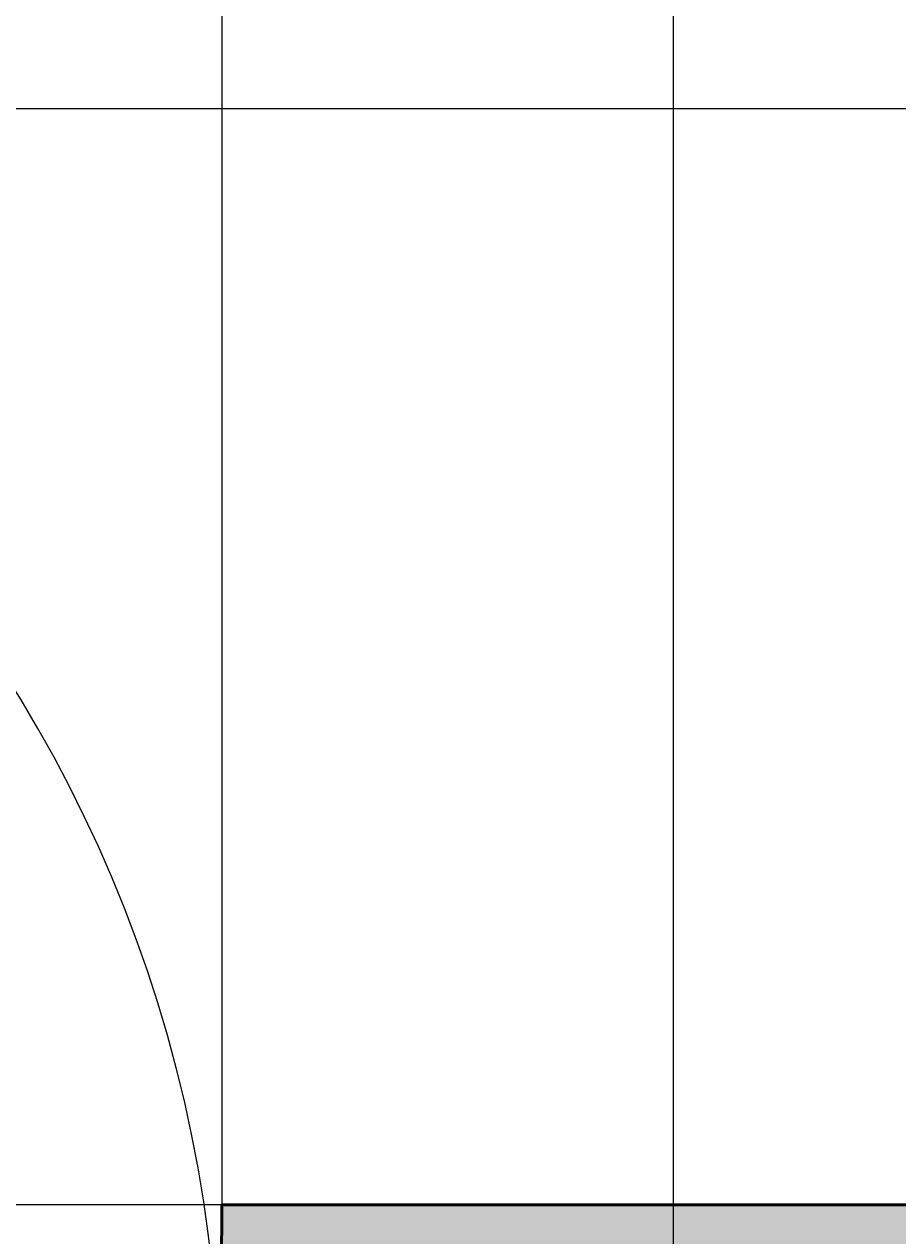
# Model space of a CAD drawing. Units: inches. Extents: x 2231 to 2461, y 2045 to 2455.
# Tile 15 of 95: x 2326 to 2346, y 2072 to 2099. Entities that reach past the tile are written whole.
import ezdxf

# ---------------------------------------------------------------- set-up
doc = ezdxf.new("R2010")
doc.units = ezdxf.units.IN
for name, color, linetype, lineweight in [('A-ANNO-DIMS', 2, 'Continuous', 18), ('A-DOOR', 3, 'Continuous', 25), ('A-WALL', 7, 'Continuous', 50)]:
    doc.layers.add(name, color=color, linetype=linetype, lineweight=lineweight)
doc.layers.add('A-WALL-PATT', color=18, linetype='Continuous', lineweight=13, true_color=0x000000)
doc.styles.get("Standard").update_dxf_attribs({"font": 'arial.ttf'})
doc.dimstyles.get("Standard").update_dxf_attribs({"dimtxt": 0.18, "dimasz": 0.18, "dimexe": 0.18, "dimexo": 0.0625, "dimgap": 0.09, "dimtad": 0, "dimtih": 1, "dimtoh": 1, "dimdec": 4, "dimzin": 0, "dimdsep": 46, "dimtxsty": 'Standard', "dimcen": 0.09, "dimadec": 0, "dimazin": 0, "dimtfac": 1, "dimtdec": 4, "dimtofl": 0, "dimtmove": 0, "dimatfit": 3, "dimfxl": 1, "dimtolj": 1, "dimtzin": 0, "dimarcsym": 0})

# ---------------------------------------------------------------- blocks, each defined once
blk = doc.blocks.new('*U5')
blk.add_arc((0, 0), 40, 0, 90)
blk = doc.blocks.new('*D51')
at = {"layer": 'A-ANNO-DIMS', "color": 0, "lineweight": -2, "transparency": 16777216}
for p, q in [((2258.794, 2306.77), (2258.794, 2044.803)), ((2330.794, 2306.77), (2330.794, 2044.803)), ((2258.974, 2044.983), (2294.576, 2044.983)), ((2330.614, 2044.983), (2295.011, 2044.983))]:
    blk.add_line(p, q, dxfattribs=at)
at = {"layer": 'A-ANNO-DIMS', "color": 0, "transparency": 16777216}
for points in [[(2258.974, 2045.013), (2258.974, 2044.953), (2258.794, 2044.983)], [(2330.614, 2045.013), (2330.614, 2044.953), (2330.794, 2044.983)]]:
    blk.add_solid(points, dxfattribs=at)
at = {"layer": 'Defpoints', "color": 0, "transparency": 16777216}
for p in [(2258.794, 2306.833), (2330.794, 2306.833), (2330.794, 2044.983)]:
    blk.add_point(p, dxfattribs=at)
at = {"layer": 'A-ANNO-DIMS', "color": 0, "transparency": 16777216, "insert": (2294.794, 2044.983), "char_height": 0.18, "attachment_point": 5}
blk.add_mtext('\\A1;72', dxfattribs=at)
blk = doc.blocks.new('*D52')
at = {"layer": 'A-ANNO-DIMS', "color": 0, "lineweight": -2, "transparency": 16777216}
for p, q in [((2330.794, 2306.77), (2330.794, 2044.803)), ((2360.794, 2306.77), (2360.794, 2044.803)), ((2330.974, 2044.983), (2345.575, 2044.983)), ((2360.614, 2044.983), (2346.012, 2044.983))]:
    blk.add_line(p, q, dxfattribs=at)
at = {"layer": 'A-ANNO-DIMS', "color": 0, "transparency": 16777216}
for points in [[(2330.974, 2045.013), (2330.974, 2044.953), (2330.794, 2044.983)], [(2360.614, 2045.013), (2360.614, 2044.953), (2360.794, 2044.983)]]:
    blk.add_solid(points, dxfattribs=at)
at = {"layer": 'Defpoints', "color": 0, "transparency": 16777216}
for p in [(2330.794, 2306.833), (2360.794, 2306.833), (2360.794, 2044.983)]:
    blk.add_point(p, dxfattribs=at)
at = {"layer": 'A-ANNO-DIMS', "color": 0, "transparency": 16777216, "insert": (2345.794, 2044.983), "char_height": 0.18, "attachment_point": 5}
blk.add_mtext('\\A1;30', dxfattribs=at)
blk = doc.blocks.new('*D65')
at = {"layer": 'A-ANNO-DIMS', "color": 0, "lineweight": -2, "transparency": 16777216}
for p, q in [((2285.635, 2189.285), (2285.635, 2044.803)), ((2340.667, 2189.285), (2340.667, 2044.803)), ((2285.815, 2044.983), (2312.758, 2044.983)), ((2340.487, 2044.983), (2313.545, 2044.983))]:
    blk.add_line(p, q, dxfattribs=at)
at = {"layer": 'A-ANNO-DIMS', "color": 0, "transparency": 16777216}
for points in [[(2285.815, 2045.013), (2285.815, 2044.953), (2285.635, 2044.983)], [(2340.487, 2045.013), (2340.487, 2044.953), (2340.667, 2044.983)]]:
    blk.add_solid(points, dxfattribs=at)
at = {"layer": 'Defpoints', "color": 0, "transparency": 16777216}
for p in [(2285.635, 2189.348), (2340.667, 2189.348), (2340.667, 2044.983)]:
    blk.add_point(p, dxfattribs=at)
at = {"layer": 'A-ANNO-DIMS', "color": 0, "transparency": 16777216, "insert": (2313.151, 2044.983), "char_height": 0.18, "attachment_point": 5}
blk.add_mtext('\\A1;55.03', dxfattribs=at)
blk = doc.blocks.new('*D67')
at = {"layer": 'A-ANNO-DIMS', "color": 0, "lineweight": -2, "transparency": 16777216}
for p, q in [((2348.126, 2096.833), (2230.981, 2096.833)), ((2231.161, 2096.653), (2231.161, 2085.013)), ((2231.161, 2073.013), (2231.161, 2084.652)), ((2348.559, 2072.833), (2230.981, 2072.833))]:
    blk.add_line(p, q, dxfattribs=at)
at = {"layer": 'A-ANNO-DIMS', "color": 0, "transparency": 16777216}
for points in [[(2231.131, 2096.653), (2231.191, 2096.653), (2231.161, 2096.833)], [(2231.131, 2073.013), (2231.191, 2073.013), (2231.161, 2072.833)]]:
    blk.add_solid(points, dxfattribs=at)
at = {"layer": 'Defpoints', "color": 0, "transparency": 16777216}
for p in [(2348.189, 2096.833), (2231.161, 2072.833), (2348.622, 2072.833)]:
    blk.add_point(p, dxfattribs=at)
at = {"layer": 'A-ANNO-DIMS', "color": 0, "transparency": 16777216, "insert": (2231.161, 2084.833), "char_height": 0.18, "attachment_point": 5}
blk.add_mtext('\\A1;24', dxfattribs=at)
blk = doc.blocks.new('*D69')
at = {"layer": 'A-ANNO-DIMS', "color": 0, "lineweight": -2, "transparency": 16777216}
for p, q in [((2340.667, 2189.285), (2340.667, 2044.803)), ((2394.794, 2186.77), (2394.794, 2044.803)), ((2340.847, 2044.983), (2367.337, 2044.983)), ((2394.614, 2044.983), (2368.124, 2044.983))]:
    blk.add_line(p, q, dxfattribs=at)
at = {"layer": 'A-ANNO-DIMS', "color": 0, "transparency": 16777216}
for points in [[(2340.847, 2045.013), (2340.847, 2044.953), (2340.667, 2044.983)], [(2394.614, 2045.013), (2394.614, 2044.953), (2394.794, 2044.983)]]:
    blk.add_solid(points, dxfattribs=at)
at = {"layer": 'Defpoints', "color": 0, "transparency": 16777216}
for p in [(2340.667, 2189.348), (2394.794, 2186.833), (2394.794, 2044.983)]:
    blk.add_point(p, dxfattribs=at)
at = {"layer": 'A-ANNO-DIMS', "color": 0, "transparency": 16777216, "insert": (2367.73, 2044.983), "char_height": 0.18, "attachment_point": 5}
blk.add_mtext('\\A1;54.13', dxfattribs=at)

msp = doc.modelspace()

# ---------------------------------------------------------------- hatches: boundary and pattern name
at = {"layer": 'A-WALL-PATT'}
h = msp.add_hatch(color=256, dxfattribs=at)
h.dxf.hatch_style = 1
h.paths.add_polyline_path([(2441.7935, 2269.1535), (2432.7935, 2269.1535), (2432.7935, 2186.8328), (2396.7935, 2186.8328), (2396.7935, 2286.8328), (2394.7935, 2286.8328), (2394.7935, 2186.8328), (2334.7935, 2186.8328), (2334.7935, 2182.8328), (2432.7935, 2182.8328), (2432.7935, 2072.8328), (2416.6639, 2072.8328), (2416.6639, 2063.8328), (2441.7935, 2063.8328)])
h.paths.add_polyline_path([(2368.6639, 2072.8328), (2367.04, 2072.8328), (2330.7942, 2072.8328), (2330.7397, 2063.8328), (2368.6639, 2063.8328)])
h.paths.add_polyline_path([(2300.7392, 2068.3328), (2300.7392, 2072.8328), (2298.7935, 2072.8328), (2294.7935, 2072.8328), (2258.7935, 2072.8328), (2258.7935, 2120.8328), (2294.7935, 2120.8328), (2298.7935, 2120.8328), (2298.7935, 2128.8328), (2294.7935, 2128.8328), (2294.7935, 2124.8328), (2258.7935, 2124.8328), (2258.7935, 2182.8328), (2294.7935, 2182.8328), (2294.7935, 2174.8328), (2298.7935, 2174.8328), (2298.7935, 2182.8328), (2304.7935, 2182.8328), (2304.7935, 2186.8328), (2258.7935, 2186.8328), (2258.7935, 2221.999), (2249.7935, 2221.999), (2249.7935, 2063.8328), (2300.7392, 2063.8328)])
h.paths.add_polyline_path([(2391.9338, 2435.8328), (2333.82, 2435.8328), (2333.82, 2426.8328), (2368.7935, 2426.8328), (2368.7935, 2374.9508), (2368.7935, 2370.8328), (2372.3935, 2370.8328), (2372.7935, 2370.8328), (2372.7935, 2426.8328), (2391.9338, 2426.8328)])
h.paths.add_polyline_path([(2441.7935, 2435.8328), (2415.9338, 2435.8328), (2415.9338, 2426.8328), (2432.7935, 2426.8328), (2432.7935, 2334.8328), (2372.7935, 2334.8328), (2372.7935, 2346.8328), (2368.7935, 2346.8328), (2368.7935, 2306.8328), (2360.7935, 2306.8328), (2360.7935, 2302.8328), (2368.7935, 2302.8328), (2372.7935, 2302.8328), (2372.7935, 2330.8328), (2432.7935, 2330.8328), (2432.7935, 2317.1535), (2441.7935, 2317.1535)])
h.paths.add_polyline_path([(2285.82, 2435.8328), (2249.7935, 2435.8328), (2249.7935, 2269.999), (2258.7935, 2269.999), (2258.7935, 2302.8328), (2318.8168, 2302.8328), (2330.7935, 2302.8328), (2330.7935, 2306.8328), (2258.7935, 2306.8328), (2258.7935, 2426.8328), (2285.82, 2426.8328)])

# ---------------------------------------------------------------- linework, layer by layer
at = {"layer": 'A-WALL'}
for p, q in [((2330.7942, 2072.8328), (2330.7384, 2063.615)), ((2432.7935, 2072.8328), (2330.7942, 2072.8328))]:
    msp.add_line(p, q, dxfattribs=at)

# ---------------------------------------------------------------- block references
at = {"layer": 'A-DOOR', "xscale": 0.75, "yscale": 0.75, "zscale": 0.75}
msp.add_blockref('*U5', (2300.7392, 2068.3328), dxfattribs=at)

# ---------------------------------------------------------------- dimensions: what is measured, and where the dimension line sits
at = {"layer": 'A-ANNO-DIMS'}
for base, p1, p2, override, picture, middle in [((2330.7935, 2044.9825), (2258.7935, 2306.8328), (2330.7935, 2306.8328), {"dimdec": 0, "dimlfac": 1, "dimrnd": 0, "dimzin": 0, "dimdsep": 46, "dimlunit": 2}, '*D51', (2294.7935, 2044.9825)), ((2360.7935, 2044.9825), (2330.7935, 2306.8328), (2360.7935, 2306.8328), {"dimdec": 0, "dimlfac": 1, "dimrnd": 0, "dimzin": 0, "dimdsep": 46, "dimlunit": 2}, '*D52', (2345.7935, 2044.9825)), ((2340.6673, 2044.9825), (2285.6353, 2189.3477), (2340.6673, 2189.3477), {"dimdec": 2, "dimlfac": 1, "dimrnd": 0, "dimzin": 0, "dimdsep": 46, "dimlunit": 2}, '*D65', (2313.1513, 2044.9825)), ((2394.7935, 2044.9825), (2340.6673, 2189.3477), (2394.7935, 2186.8328), {"dimdec": 2, "dimlfac": 1, "dimrnd": 0, "dimzin": 0, "dimdsep": 46, "dimlunit": 2}, '*D69', (2367.7304, 2044.9825))]:
    dim = msp.add_linear_dim(base=base, p1=p1, p2=p2, dimstyle='Standard', override=override, dxfattribs=at)
    dim.commit()
    dim.dimension.update_dxf_attribs({"geometry": picture, "text_midpoint": middle})
dim = msp.add_linear_dim(base=(2231.161, 2072.8328), p1=(2348.1888, 2096.8328), p2=(2348.6219, 2072.8328), angle=90, dimstyle='Standard', override={"dimdec": 0, "dimlfac": 1, "dimrnd": 0, "dimzin": 0, "dimdsep": 46, "dimlunit": 2}, dxfattribs=at)
dim.commit()
dim.dimension.update_dxf_attribs({"geometry": '*D67', "text_midpoint": (2231.161, 2084.8328)})

doc.saveas('drawing.dxf')
